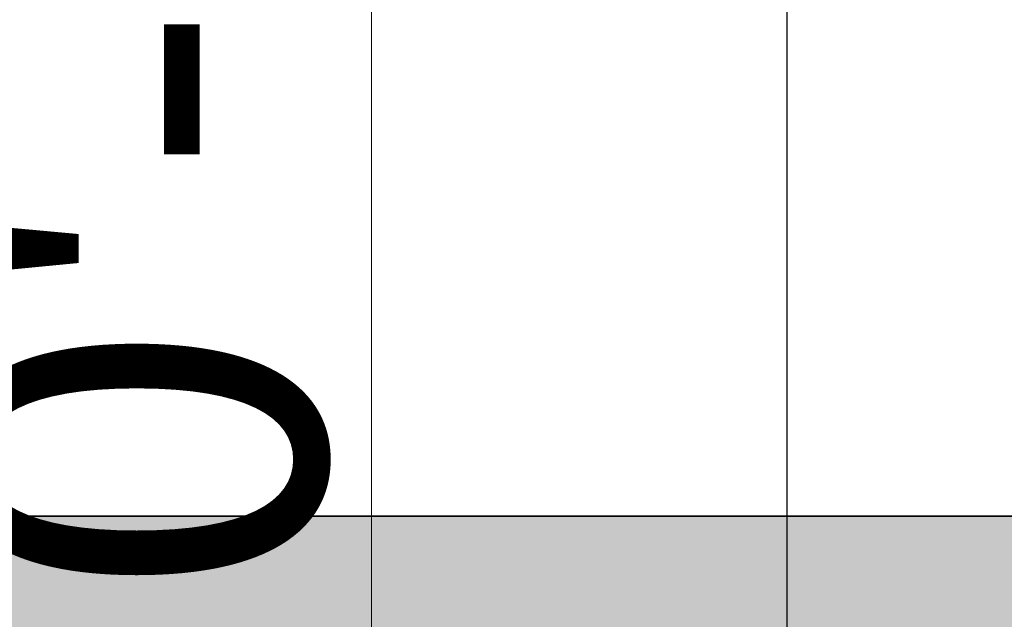
# Model space of a CAD drawing. Units: inches. Extents: x 2696 to 3240, y 1564 to 2310.
# Tile 47 of 76: x 2770.48 to 2786.34, y 2094.04 to 2103.71. Entities that reach past the tile are written whole.
import ezdxf

# ---------------------------------------------------------------- set-up
doc = ezdxf.new("R2010")
doc.units = ezdxf.units.IN
for name, color, linetype, lineweight in [('A-ANNO-DIMS', 3, 'Continuous', 18), ('A-WALL', 7, 'Continuous', 35), ('A-WALL-PATT', 9, 'Continuous', 13)]:
    doc.layers.add(name, color=color, linetype=linetype, lineweight=lineweight)
doc.styles.add('TIMES NEW', font='times.ttf')
doc.dimstyles.new('Siddhuu', dxfattribs={"dimtxt": 6, "dimasz": 2.5, "dimexe": 1.25, "dimexo": 0.625, "dimtad": 1, "dimdec": 1, "dimlunit": 4, "dimtxsty": 'TIMES NEW', "dimcen": 2.5, "dimclrd": 256, "dimclre": 1, "dimclrt": 7, "dimadec": 0, "dimazin": 0, "dimtfac": 1, "dimtdec": 1, "dimtmove": 0, "dimatfit": 3, "dimfxl": 1, "dimtolj": 1, "dimlwd": -1, "dimarcsym": 0})

# ---------------------------------------------------------------- blocks, each defined once
blk = doc.blocks.new('*D40')
at = {"layer": 'A-ANNO-DIMS', "color": 1, "lineweight": -2, "transparency": 16777216}
for p, q in [((2777.266, 2091.826), (2777.266, 2093.576)), ((2784.764, 2091.826), (2784.764, 2093.576))]:
    blk.add_line(p, q, dxfattribs=at)
at = {"layer": 'A-ANNO-DIMS', "transparency": 16777216}
for p, q in [((2779.766, 2092.326), (2782.264, 2092.326)), ((2784.764, 2092.326), (2902.458, 2092.326))]:
    blk.add_line(p, q, dxfattribs=at)
for points in [[(2779.766, 2092.742), (2779.766, 2091.909), (2777.266, 2092.326)], [(2782.264, 2092.742), (2782.264, 2091.909), (2784.764, 2092.326)]]:
    blk.add_solid(points, dxfattribs=at)
at = {"layer": 'Defpoints', "color": 0, "transparency": 16777216}
for p in [(2784.764, 2092.326), (2777.266, 2091.201), (2784.764, 2091.201)]:
    blk.add_point(p, dxfattribs=at)
at = {"layer": 'A-ANNO-DIMS', "color": 7, "transparency": 16777216, "insert": (2844.861, 2096.094), "char_height": 6, "attachment_point": 5, "style": 'TIMES NEW'}
blk.add_mtext('\\A1;BATH FITTING 0\'-7 1/2" TYP.', dxfattribs=at)
blk = doc.blocks.new('*D41')
at = {"layer": 'A-ANNO-DIMS', "transparency": 16777216}
for p, q in [((2776.142, 2091.201), (2776.142, 2145.728)), ((2776.142, 2087.2), (2776.142, 2088.701))]:
    blk.add_line(p, q, dxfattribs=at)
at = {"layer": 'A-ANNO-DIMS', "color": 1, "lineweight": -2, "transparency": 16777216}
for p, q in [((2776.641, 2091.201), (2774.892, 2091.201)), ((2776.641, 2084.7), (2774.892, 2084.7))]:
    blk.add_line(p, q, dxfattribs=at)
at = {"layer": 'A-ANNO-DIMS', "transparency": 16777216}
for points in [[(2775.725, 2088.701), (2776.558, 2088.701), (2776.142, 2091.201)], [(2775.725, 2087.2), (2776.558, 2087.2), (2776.142, 2084.7)]]:
    blk.add_solid(points, dxfattribs=at)
at = {"layer": 'Defpoints', "color": 0, "transparency": 16777216}
for p in [(2776.142, 2091.201), (2777.266, 2091.201), (2777.266, 2084.7)]:
    blk.add_point(p, dxfattribs=at)
at = {"layer": 'A-ANNO-DIMS', "color": 7, "transparency": 16777216, "insert": (2772.38, 2119.715), "char_height": 6, "attachment_point": 5, "rotation": 90, "style": 'TIMES NEW'}
blk.add_mtext('\\A1;0\'-6 1/2" TYP.', dxfattribs=at)
blk = doc.blocks.new('*D62')
at = {"layer": 'A-ANNO-DIMS', "color": 1, "lineweight": -2, "transparency": 16777216}
for p, q in [((2965.084, 2140.701), (2709.361, 2140.701)), ((2965.084, 2063.591), (2709.361, 2063.591))]:
    blk.add_line(p, q, dxfattribs=at)
at = {"layer": 'A-ANNO-DIMS', "transparency": 16777216}
blk.add_line((2710.611, 2066.091), (2710.611, 2138.201), dxfattribs=at)
for points in [[(2710.195, 2138.201), (2711.028, 2138.201), (2710.611, 2140.701)], [(2710.195, 2066.091), (2711.028, 2066.091), (2710.611, 2063.591)]]:
    blk.add_solid(points, dxfattribs=at)
at = {"layer": 'Defpoints', "color": 0, "transparency": 16777216}
for p in [(2710.611, 2140.701), (2965.709, 2140.701), (2965.709, 2063.591)]:
    blk.add_point(p, dxfattribs=at)
at = {"layer": 'A-ANNO-DIMS', "color": 7, "transparency": 16777216, "insert": (2706.934, 2102.146), "char_height": 6, "attachment_point": 5, "rotation": 90, "style": 'TIMES NEW'}
blk.add_mtext('\\A1;6\'-5"', dxfattribs=at)
blk = doc.blocks.new('*D64')
at = {"layer": 'A-ANNO-DIMS', "color": 1, "lineweight": -2, "transparency": 16777216}
for p, q in [((3073.084, 2206.701), (2709.361, 2206.701)), ((3068.584, 1989.201), (2709.361, 1989.201))]:
    blk.add_line(p, q, dxfattribs=at)
at = {"layer": 'A-ANNO-DIMS', "transparency": 16777216}
blk.add_line((2710.611, 1991.701), (2710.611, 2204.201), dxfattribs=at)
for points in [[(2710.195, 2204.201), (2711.028, 2204.201), (2710.611, 2206.701)], [(2710.195, 1991.701), (2711.028, 1991.701), (2710.611, 1989.201)]]:
    blk.add_solid(points, dxfattribs=at)
at = {"layer": 'Defpoints', "color": 0, "transparency": 16777216}
for p in [(2710.611, 2206.701), (3073.709, 2206.701), (3069.209, 1989.201)]:
    blk.add_point(p, dxfattribs=at)
at = {"layer": 'A-ANNO-DIMS', "color": 7, "transparency": 16777216, "insert": (2706.85, 2097.951), "char_height": 6, "attachment_point": 5, "rotation": 90, "style": 'TIMES NEW'}
blk.add_mtext('\\A1;18\'-1 1/2"', dxfattribs=at)
blk = doc.blocks.new('*D66')
at = {"layer": 'A-ANNO-DIMS', "color": 1, "lineweight": -2, "transparency": 16777216}
for p, q in [((3077.584, 2122.701), (2709.361, 2122.701)), ((3077.584, 2074.701), (2709.361, 2074.701))]:
    blk.add_line(p, q, dxfattribs=at)
at = {"layer": 'A-ANNO-DIMS', "transparency": 16777216}
blk.add_line((2710.611, 2077.201), (2710.611, 2120.201), dxfattribs=at)
for points in [[(2710.195, 2120.201), (2711.028, 2120.201), (2710.611, 2122.701)], [(2710.195, 2077.201), (2711.028, 2077.201), (2710.611, 2074.701)]]:
    blk.add_solid(points, dxfattribs=at)
at = {"layer": 'Defpoints', "color": 0, "transparency": 16777216}
for p in [(2710.611, 2122.701), (3078.209, 2122.701), (3078.209, 2074.701)]:
    blk.add_point(p, dxfattribs=at)
at = {"layer": 'A-ANNO-DIMS', "color": 7, "transparency": 16777216, "insert": (2706.934, 2098.701), "char_height": 6, "attachment_point": 5, "rotation": 90, "style": 'TIMES NEW'}
blk.add_mtext('\\A1;4\'-0"', dxfattribs=at)
blk = doc.blocks.new('*D68')
at = {"layer": 'A-ANNO-DIMS', "color": 1, "lineweight": -2, "transparency": 16777216}
for p, q in [((2745.611, 2261.576), (2745.611, 1568.951)), ((2782.834, 2261.576), (2782.834, 1568.951))]:
    blk.add_line(p, q, dxfattribs=at)
at = {"layer": 'A-ANNO-DIMS', "transparency": 16777216}
blk.add_line((2748.111, 1570.201), (2780.334, 1570.201), dxfattribs=at)
for points in [[(2748.111, 1570.618), (2748.111, 1569.784), (2745.611, 1570.201)], [(2780.334, 1570.618), (2780.334, 1569.784), (2782.834, 1570.201)]]:
    blk.add_solid(points, dxfattribs=at)
at = {"layer": 'Defpoints', "color": 0, "transparency": 16777216}
for p in [(2745.611, 2262.201), (2782.834, 2262.201), (2782.834, 1570.201)]:
    blk.add_point(p, dxfattribs=at)
at = {"layer": 'A-ANNO-DIMS', "color": 7, "transparency": 16777216, "insert": (2764.223, 1573.878), "char_height": 6, "attachment_point": 5, "style": 'TIMES NEW'}
blk.add_mtext('\\A1;3\'-1"', dxfattribs=at)

msp = doc.modelspace()

# ---------------------------------------------------------------- hatches: boundary and pattern name
at = {"layer": 'A-WALL-PATT', "transparency": 33554556}
h = msp.add_hatch(color=256, dxfattribs=at)
h.dxf.hatch_style = 1
h.paths.add_polyline_path([(2879.111, 2253.201), (2905.91, 2253.201), (2905.91, 2262.201), (2841.889, 2262.201), (2841.889, 2253.201), (2870.111, 2253.201), (2870.111, 2176.601), (2965.709, 2176.601), (2965.709, 2206.701), (2973.583, 2206.701), (2973.583, 2215.701), (2965.709, 2215.701), (2965.709, 2262.201), (2929.91, 2262.201), (2929.91, 2253.201), (2956.709, 2253.201), (2956.709, 2185.601), (2879.111, 2185.601)])
h.paths.add_polyline_path([(2782.834, 2262.201), (2745.611, 2262.201), (2745.611, 2228.729), (2754.611, 2228.729), (2754.611, 2253.201), (2782.834, 2253.201)])
h.paths.add_polyline_path([(2754.611, 2136.201), (2965.709, 2136.201), (2965.709, 2145.201), (2879.111, 2145.201), (2879.111, 2147.074), (2877.34, 2147.074), (2870.111, 2147.074), (2870.111, 2145.201), (2754.611, 2145.201), (2754.611, 2169.674), (2745.611, 2169.674), (2745.611, 2000.201), (2754.611, 2000.201), (2754.611, 2019.201), (2849.083, 2019.201), (2849.083, 2023.701), (2841.209, 2023.701), (2841.209, 2051.827), (2836.709, 2051.827), (2836.709, 2023.701), (2754.611, 2023.701), (2754.611, 2091.201), (2836.709, 2091.201), (2836.709, 2087.827), (2841.209, 2087.827), (2841.209, 2095.701), (2754.611, 2095.701)])
h.paths.add_polyline_path([(2965.709, 2136.201), (2956.709, 2136.201), (2956.709, 2023.701), (2885.083, 2023.701), (2885.083, 2019.201), (2956.709, 2019.201), (2956.709, 1950.575), (2965.709, 1950.575), (2965.709, 1980.201), (2973.583, 1980.201), (2973.583, 1989.201), (2965.709, 1989.201)])
h.paths.add_polyline_path([(2754.611, 1906.701), (2880.209, 1906.701), (2884.709, 1906.701), (2956.709, 1906.701), (2956.709, 1792.701), (2944.709, 1792.701), (2944.709, 1783.701), (2956.709, 1783.701), (2956.709, 1740.201), (2884.709, 1740.201), (2884.709, 1783.701), (2896.709, 1783.701), (2896.709, 1792.701), (2884.709, 1792.701), (2884.709, 1846.701), (2880.209, 1846.701), (2880.209, 1740.201), (2754.611, 1740.201), (2754.611, 1777.201), (2745.611, 1777.201), (2745.611, 1692.701), (2754.611, 1692.701), (2754.611, 1731.201), (2956.709, 1731.201), (2956.709, 1723.327), (2965.709, 1723.327), (2965.709, 1884.201), (2973.583, 1884.201), (2973.583, 1893.201), (2965.709, 1893.201), (2965.709, 1914.575), (2956.709, 1914.575), (2956.709, 1911.201), (2754.611, 1911.201), (2754.611, 1930.201), (2745.611, 1930.201), (2745.611, 1817.201), (2754.611, 1817.201), (2754.611, 1854.201), (2826.611, 1854.201), (2826.611, 1868.827), (2822.111, 1868.827), (2822.111, 1858.701), (2754.611, 1858.701)])
h.paths.add_polyline_path([(2965.709, 1656.201), (3008.237, 1656.201), (3008.237, 1665.201), (2965.709, 1665.201), (2965.709, 1693.327), (2956.709, 1693.327), (2956.709, 1686.201), (2934.583, 1686.201), (2934.583, 1681.701), (2956.709, 1681.701), (2956.709, 1614.201), (2896.709, 1614.201), (2896.709, 1681.701), (2904.583, 1681.701), (2904.583, 1686.201), (2892.209, 1686.201), (2892.209, 1614.201), (2858.41, 1614.201), (2858.41, 1605.201), (2965.709, 1605.201)])
h.paths.add_polyline_path([(2788.41, 1614.201), (2754.611, 1614.201), (2754.611, 1652.701), (2745.611, 1652.701), (2745.611, 1605.201), (2788.41, 1605.201)])
h.paths.add_polyline_path([(3199.611, 1633.048), (3190.611, 1633.048), (3190.611, 1614.201), (3082.611, 1614.201), (3082.611, 1665.201), (3070.237, 1665.201), (3070.237, 1656.201), (3078.111, 1656.201), (3078.111, 1605.201), (3199.611, 1605.201)])
h.paths.add_polyline_path([(3199.611, 1702.048), (3190.611, 1702.048), (3190.611, 1699.701), (3106.611, 1699.701), (3106.611, 1747.701), (3190.611, 1747.701), (3190.611, 1752.201), (3082.611, 1752.201), (3082.611, 1760.075), (3078.111, 1760.075), (3078.111, 1747.701), (3102.111, 1747.701), (3102.111, 1699.701), (3078.111, 1699.701), (3078.111, 1695.201), (3190.611, 1695.201), (3190.611, 1676.355), (3199.611, 1676.355)])
h.paths.add_polyline_path([(3199.611, 1783.201), (3190.611, 1783.201), (3190.611, 1745.355), (3199.611, 1745.355)])
h.paths.add_polyline_path([(3082.611, 1884.201), (3190.611, 1884.201), (3190.611, 1853.201), (3199.611, 1853.201), (3199.611, 1901.701), (3190.611, 1901.701), (3190.611, 1893.201), (3005.583, 1893.201), (3005.583, 1891.281), (3005.583, 1884.201), (3078.111, 1884.201), (3078.111, 1792.075), (3082.611, 1792.075)])
h.paths.add_polyline_path([(3199.611, 1994.701), (3190.611, 1994.701), (3190.611, 1989.201), (3073.709, 1989.201), (3073.709, 2034.201), (3069.209, 2034.201), (3069.209, 1989.201), (3005.583, 1989.201), (3005.583, 1980.201), (3190.611, 1980.201), (3190.611, 1971.701), (3199.611, 1971.701)])
h.paths.add_polyline_path([(3199.611, 2155.201), (3190.611, 2155.201), (3190.611, 2064.701), (3199.611, 2064.701)])
h.paths.add_polyline_path([(3190.611, 2074.701), (3106.611, 2074.701), (3106.611, 2122.701), (3190.611, 2122.701), (3190.611, 2127.201), (3082.709, 2127.201), (3082.709, 2135.075), (3073.709, 2135.075), (3073.709, 2122.701), (3102.111, 2122.701), (3102.111, 2074.701), (3069.209, 2074.701), (3069.209, 2070.201), (3190.611, 2070.201)])
h.paths.add_polyline_path([(3082.709, 2253.201), (3190.611, 2253.201), (3190.611, 2225.201), (3199.611, 2225.201), (3199.611, 2262.201), (3073.709, 2262.201), (3073.709, 2215.701), (3035.583, 2215.701), (3035.583, 2206.701), (3073.709, 2206.701), (3073.709, 2171.075), (3082.709, 2171.075)])

# ---------------------------------------------------------------- linework, layer by layer
at = {"layer": 'A-WALL'}
msp.add_line((2754.611, 2095.701), (2841.209, 2095.701), dxfattribs=at)

# ---------------------------------------------------------------- dimensions: what is measured, and where the dimension line sits
at = {"layer": 'A-ANNO-DIMS'}
dim = msp.add_linear_dim(base=(2782.834, 1570.201), p1=(2745.611, 2262.201), p2=(2782.834, 2262.201), dimstyle='Siddhuu', override={"dimdec": 1, "dimlfac": 1, "dimrnd": 0, "dimzin": 1, "dimdsep": 46, "dimlunit": 4, "dimfrac": 2}, dxfattribs=at)
dim.commit()
dim.dimension.update_dxf_attribs({"geometry": '*D68', "text_midpoint": (2764.223, 1573.878)})
for base, p1, p2, picture, middle in [((2710.611, 2206.701), (3069.209, 1989.201), (3073.709, 2206.701), '*D64', (2706.85, 2097.951)), ((2710.611, 2140.701), (2965.709, 2063.591), (2965.709, 2140.701), '*D62', (2706.934, 2102.146)), ((2710.611, 2122.701), (3078.209, 2074.701), (3078.209, 2122.701), '*D66', (2706.934, 2098.701))]:
    dim = msp.add_linear_dim(base=base, p1=p1, p2=p2, angle=90, dimstyle='Siddhuu', override={"dimdec": 1, "dimlfac": 1, "dimrnd": 0, "dimzin": 1, "dimdsep": 46, "dimlunit": 4, "dimfrac": 2}, dxfattribs=at)
    dim.commit()
    dim.dimension.update_dxf_attribs({"geometry": picture, "text_midpoint": middle})
dim = msp.add_linear_dim(base=(2776.142, 2091.201), p1=(2777.266, 2084.7), p2=(2777.266, 2091.201), angle=90, text='<> TYP.', dimstyle='Siddhuu', override={"dimdec": 1, "dimlfac": 1, "dimrnd": 0, "dimzin": 1, "dimdsep": 46, "dimlunit": 4, "dimfrac": 2}, dxfattribs=at)
dim.commit()
dim.dimension.update_dxf_attribs({"geometry": '*D41', "text_midpoint": (2772.38, 2119.715)})
dim = msp.add_linear_dim(base=(2784.764, 2092.326), p1=(2777.266, 2091.201), p2=(2784.764, 2091.201), text='BATH FITTING <> TYP.', dimstyle='Siddhuu', override={"dimdec": 1, "dimlfac": 1, "dimrnd": 0, "dimzin": 1, "dimdsep": 46, "dimlunit": 4, "dimfrac": 2}, dxfattribs=at)
dim.commit()
dim.dimension.update_dxf_attribs({"geometry": '*D40', "text_midpoint": (2844.861, 2096.094)})

doc.saveas('drawing.dxf')
